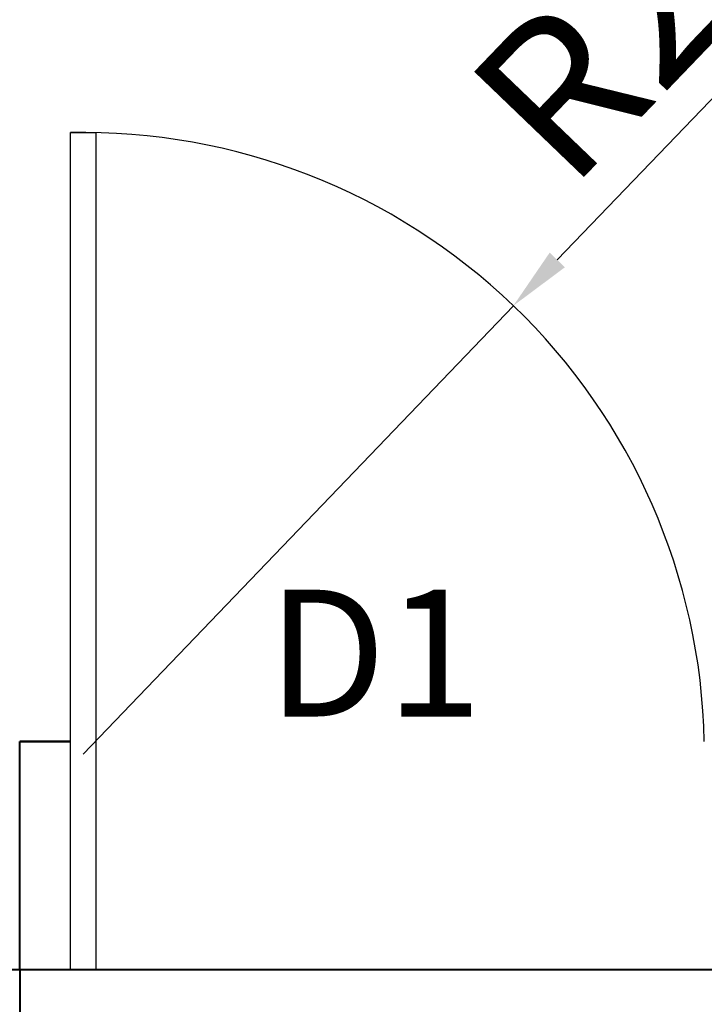
# Model space of a CAD drawing. Units: inches. Extents: x 459864 to 460310, y 324185 to 324787.
# Tile 63 of 112: x 460061 to 460088, y 324282 to 324321. Entities that reach past the tile are written whole.
import ezdxf

# ---------------------------------------------------------------- set-up
doc = ezdxf.new("R2010")
doc.units = ezdxf.units.IN
for name, color, linetype, lineweight in [('A-ANNO-DIMS', 2, 'Continuous', 18), ('A-ANNO-TEXT', 7, 'Continuous', 18), ('A-DOOR', 3, 'Continuous', 25), ('A-WALL', 7, 'Continuous', 40), ('L-SITE-PATT', 252, 'Continuous', 13)]:
    doc.layers.add(name, color=color, linetype=linetype, lineweight=lineweight)
doc.styles.get("Standard").update_dxf_attribs({"font": 'arial.ttf'})
doc.dimstyles.new('ISO-25', dxfattribs={"dimtxt": 6, "dimasz": 2.5, "dimexe": 1.25, "dimexo": 0.625, "dimtad": 1, "dimdec": 1, "dimlunit": 3, "dimtxsty": 'Standard', "dimcen": 2.5, "dimadec": 0, "dimazin": 0, "dimtfac": 1, "dimtdec": 1, "dimtmove": 0, "dimatfit": 3, "dimfxl": 1, "dimarcsym": 0})

# ---------------------------------------------------------------- blocks, each defined once
blk = doc.blocks.new('*D69')
at = {"layer": 'A-ANNO-DIMS', "color": 0, "lineweight": -2, "transparency": 16777216}
for p, q in [((460055.99, 324376.483), (459874.965, 324376.483)), ((459876.215, 324373.983), (459876.215, 324285.983)), ((460060.49, 324283.483), (459874.965, 324283.483))]:
    blk.add_line(p, q, dxfattribs=at)
at = {"layer": 'A-ANNO-DIMS', "color": 0, "transparency": 16777216}
for points in [[(459875.798, 324373.983), (459876.632, 324373.983), (459876.215, 324376.483)], [(459875.798, 324285.983), (459876.632, 324285.983), (459876.215, 324283.483)]]:
    blk.add_solid(points, dxfattribs=at)
at = {"layer": 'Defpoints', "color": 0, "transparency": 16777216}
for p in [(460056.615, 324376.483), (459876.215, 324283.483), (460061.115, 324283.483)]:
    blk.add_point(p, dxfattribs=at)
at = {"layer": 'A-ANNO-DIMS', "color": 0, "transparency": 16777216, "insert": (459872.526, 324329.983), "char_height": 6, "attachment_point": 5, "rotation": 90}
blk.add_mtext('7\'-9"', dxfattribs=at)
blk = doc.blocks.new('*D73')
at = {"layer": 'A-ANNO-DIMS', "color": 0, "lineweight": -2, "transparency": 16777216}
for p, q in [((460109.617, 324339.904), (460082.316, 324311.465)), ((460063.615, 324291.983), (460080.585, 324309.661))]:
    blk.add_line(p, q, dxfattribs=at)
at = {"layer": 'A-ANNO-DIMS', "color": 0, "transparency": 16777216}
blk.add_solid([(460082.016, 324311.753), (460082.617, 324311.176), (460080.585, 324309.661)], dxfattribs=at)
at = {"layer": 'Defpoints', "color": 0, "transparency": 16777216}
for p in [(460080.585, 324309.661), (460063.615, 324291.983)]:
    blk.add_point(p, dxfattribs=at)
at = {"layer": 'A-ANNO-DIMS', "color": 0, "transparency": 16777216, "insert": (460094.144, 324329.167), "char_height": 6, "attachment_point": 5, "rotation": 46.1701}
blk.add_mtext('R2\'-0 1/2"', dxfattribs=at)

msp = doc.modelspace()

# ---------------------------------------------------------------- hatches: boundary and pattern name
at = {"layer": 'L-SITE-PATT'}
h = msp.add_hatch(dxfattribs=at)
h.set_pattern_fill('DOTS', color=256)
h.paths.add_polyline_path([(460269.804, 324283.483), (460247.115, 324283.483), (460121.929, 324283.483), (460121.929, 324252.473), (460117.429, 324252.473), (460110.124, 324252.473), (460110.124, 324243.287), (460080.83, 324243.287), (460080.83, 324252.473), (460061.115, 324252.473), (460061.115, 324251.882), (460077.909, 324251.882), (460077.909, 324199.483), (460080.83, 324199.483), (460080.83, 324207.553), (460110.124, 324207.553), (460110.124, 324199.483), (460110.813, 324199.483), (460262.115, 324199.483), (460269.804, 324199.483)], flags=17)
edge = h.paths.add_edge_path(flags=0)
edge.add_ellipse((460222.59, 324263.813), major_axis=(-8.485, 8.485), ratio=1, start_angle=405, end_angle=495, ccw=False)
edge.add_line((460214.821, 324254.66), (460214.832, 324254.666))
edge.add_ellipse((460222.59, 324263.813), major_axis=(-8.485, 8.485), ratio=1, start_angle=405, end_angle=495, ccw=False)
edge.add_line((460210.759, 324261.781), (460210.768, 324261.787))
edge.add_ellipse((460222.59, 324263.813), major_axis=(-8.485, 8.485), ratio=1, start_angle=405, end_angle=495, ccw=False)
edge.add_ellipse((460222.59, 324263.813), major_axis=(-8.485, 8.485), ratio=1, start_angle=392.754, end_angle=405, ccw=False)
edge.add_ellipse((460222.59, 324263.813), major_axis=(-8.485, 8.485), ratio=1, start_angle=380.9347, end_angle=392.754, ccw=False)
edge.add_line((460211.337, 324267.985), (460211.34, 324267.985))
edge.add_ellipse((460222.59, 324263.813), major_axis=(-8.485, 8.485), ratio=1, start_angle=380.9347, end_angle=392.754, ccw=False)
edge.add_ellipse((460222.59, 324263.813), major_axis=(-8.485, 8.485), ratio=1, start_angle=347.9015, end_angle=380.9347, ccw=False)
edge.add_ellipse((460222.59, 324263.813), major_axis=(-8.485, 8.485), ratio=1, start_angle=327.0619, end_angle=347.9015, ccw=False)
edge.add_ellipse((460222.59, 324263.813), major_axis=(-8.485, 8.485), ratio=1, start_angle=278.3246, end_angle=327.0619, ccw=False)
edge.add_line((460225.158, 324275.536), (460225.158, 324275.535))
edge.add_ellipse((460222.59, 324263.813), major_axis=(-8.485, 8.485), ratio=1, start_angle=278.3246, end_angle=327.0619, ccw=False)
edge.add_ellipse((460222.59, 324263.813), major_axis=(-8.485, 8.485), ratio=1, start_angle=260.6436, end_angle=278.3246, ccw=False)
edge.add_ellipse((460222.59, 324263.813), major_axis=(-8.485, 8.485), ratio=1, start_angle=225, end_angle=260.6436, ccw=False)
edge.add_line((460234.509, 324265.243), (460234.501, 324265.239))
edge.add_ellipse((460222.59, 324263.813), major_axis=(-8.485, 8.485), ratio=1, start_angle=225, end_angle=260.6436, ccw=False)
edge.add_ellipse((460222.59, 324263.813), major_axis=(-8.485, 8.485), ratio=1, start_angle=495, end_angle=585, ccw=False)
edge.add_line((460234.437, 324261.861), (460234.424, 324261.858))
edge.add_ellipse((460222.59, 324263.813), major_axis=(-8.485, 8.485), ratio=1, start_angle=495, end_angle=585, ccw=False)
edge.add_line((460227.95, 324253.067), (460227.946, 324253.083))
edge.add_ellipse((460222.59, 324263.813), major_axis=(-8.485, 8.485), ratio=1, start_angle=495, end_angle=585, ccw=False)
edge.add_line((460226.223, 324252.369), (460226.211, 324252.38))
edge.add_ellipse((460222.59, 324263.813), major_axis=(-8.485, 8.485), ratio=1, start_angle=495, end_angle=585, ccw=False)
h.paths.add_polyline_path([(460219.651, 324254.347), (460218.461, 324253.545), (460218.275, 324254.789), (460219.642, 324256.542), (460219.625, 324260.848), (460216.11, 324257.333), (460214.35, 324256.978), (460215.416, 324259.356), (460212.524, 324258.496), (460213.137, 324259.93), (460218.507, 324263.813), (460222.59, 324263.813), (460222.59, 324267.807), (460218.176, 324272.212), (460219.026, 324274.639), (460222.59, 324272.811), (460222.59, 324275.423), (460223.057, 324274.825), (460222.675, 324273.492), (460225.912, 324267.135), (460219.625, 324260.848)], flags=0)
edge = h.paths.add_edge_path(flags=0)
edge.add_ellipse((460194.576, 324264.046), major_axis=(-8.485, 8.485), ratio=1, start_angle=495, end_angle=585, ccw=False)
edge.add_line((460199.936, 324253.3), (460199.932, 324253.316))
edge.add_ellipse((460194.576, 324264.046), major_axis=(-8.485, 8.485), ratio=1, start_angle=495, end_angle=585, ccw=False)
edge.add_line((460198.208, 324252.603), (460198.196, 324252.613))
edge.add_ellipse((460194.576, 324264.046), major_axis=(-8.485, 8.485), ratio=1, start_angle=495, end_angle=585, ccw=False)
edge.add_ellipse((460194.576, 324264.046), major_axis=(-8.485, 8.485), ratio=1, start_angle=405, end_angle=495, ccw=False)
edge.add_line((460186.806, 324254.893), (460186.817, 324254.899))
edge.add_ellipse((460194.576, 324264.046), major_axis=(-8.485, 8.485), ratio=1, start_angle=405, end_angle=495, ccw=False)
edge.add_line((460182.744, 324262.014), (460182.753, 324262.02))
edge.add_ellipse((460194.576, 324264.046), major_axis=(-8.485, 8.485), ratio=1, start_angle=405, end_angle=495, ccw=False)
edge.add_ellipse((460194.576, 324264.046), major_axis=(-8.485, 8.485), ratio=1, start_angle=392.754, end_angle=405, ccw=False)
edge.add_ellipse((460194.576, 324264.046), major_axis=(-8.485, 8.485), ratio=1, start_angle=380.9347, end_angle=392.754, ccw=False)
edge.add_line((460183.323, 324268.218), (460183.326, 324268.218))
edge.add_ellipse((460194.576, 324264.046), major_axis=(-8.485, 8.485), ratio=1, start_angle=380.9347, end_angle=392.754, ccw=False)
edge.add_ellipse((460194.576, 324264.046), major_axis=(-8.485, 8.485), ratio=1, start_angle=347.9015, end_angle=380.9347, ccw=False)
edge.add_ellipse((460194.576, 324264.046), major_axis=(-8.485, 8.485), ratio=1, start_angle=327.0619, end_angle=347.9015, ccw=False)
edge.add_ellipse((460194.576, 324264.046), major_axis=(-8.485, 8.485), ratio=1, start_angle=278.3246, end_angle=327.0619, ccw=False)
edge.add_line((460197.144, 324275.769), (460197.143, 324275.768))
edge.add_ellipse((460194.576, 324264.046), major_axis=(-8.485, 8.485), ratio=1, start_angle=278.3246, end_angle=327.0619, ccw=False)
edge.add_ellipse((460194.576, 324264.046), major_axis=(-8.485, 8.485), ratio=1, start_angle=260.6436, end_angle=278.3246, ccw=False)
edge.add_ellipse((460194.576, 324264.046), major_axis=(-8.485, 8.485), ratio=1, start_angle=225, end_angle=260.6436, ccw=False)
edge.add_line((460206.494, 324265.476), (460206.487, 324265.473))
edge.add_ellipse((460194.576, 324264.046), major_axis=(-8.485, 8.485), ratio=1, start_angle=225, end_angle=260.6436, ccw=False)
edge.add_ellipse((460194.576, 324264.046), major_axis=(-8.485, 8.485), ratio=1, start_angle=495, end_angle=585, ccw=False)
edge.add_line((460206.422, 324262.094), (460206.409, 324262.091))
h.paths.add_polyline_path([(460191.61, 324261.081), (460191.637, 324254.58), (460190.447, 324253.778), (460190.261, 324255.023), (460191.628, 324256.775), (460191.61, 324261.081), (460188.096, 324257.566), (460186.335, 324257.211), (460187.402, 324259.589), (460184.509, 324258.729), (460185.123, 324260.163), (460190.493, 324264.046), (460194.576, 324264.046), (460194.576, 324268.04), (460190.161, 324272.446), (460191.011, 324274.872), (460194.576, 324273.044), (460194.576, 324275.657), (460195.043, 324275.058), (460194.661, 324273.725), (460197.897, 324267.368)], flags=0)
edge = h.paths.add_edge_path(flags=0)
edge.add_ellipse((460252.912, 324263.578), major_axis=(-8.485, 8.485), ratio=1, start_angle=405, end_angle=495, ccw=False)
edge.add_line((460241.081, 324261.545), (460241.089, 324261.551))
edge.add_ellipse((460252.912, 324263.578), major_axis=(-8.485, 8.485), ratio=1, start_angle=405, end_angle=495, ccw=False)
edge.add_ellipse((460252.912, 324263.578), major_axis=(-8.485, 8.485), ratio=1, start_angle=392.754, end_angle=405, ccw=False)
edge.add_ellipse((460252.912, 324263.578), major_axis=(-8.485, 8.485), ratio=1, start_angle=380.9347, end_angle=392.754, ccw=False)
edge.add_line((460241.659, 324267.749), (460241.662, 324267.749))
edge.add_ellipse((460252.912, 324263.578), major_axis=(-8.485, 8.485), ratio=1, start_angle=380.9347, end_angle=392.754, ccw=False)
edge.add_ellipse((460252.912, 324263.578), major_axis=(-8.485, 8.485), ratio=1, start_angle=347.9015, end_angle=380.9347, ccw=False)
edge.add_ellipse((460252.912, 324263.578), major_axis=(-8.485, 8.485), ratio=1, start_angle=327.0619, end_angle=347.9015, ccw=False)
edge.add_ellipse((460252.912, 324263.578), major_axis=(-8.485, 8.485), ratio=1, start_angle=278.3246, end_angle=327.0619, ccw=False)
edge.add_line((460255.48, 324275.3), (460255.479, 324275.299))
edge.add_ellipse((460252.912, 324263.578), major_axis=(-8.485, 8.485), ratio=1, start_angle=278.3246, end_angle=327.0619, ccw=False)
edge.add_ellipse((460252.912, 324263.578), major_axis=(-8.485, 8.485), ratio=1, start_angle=260.6436, end_angle=278.3246, ccw=False)
edge.add_ellipse((460252.912, 324263.578), major_axis=(-8.485, 8.485), ratio=1, start_angle=225, end_angle=260.6436, ccw=False)
edge.add_line((460264.83, 324265.007), (460264.823, 324265.004))
edge.add_ellipse((460252.912, 324263.578), major_axis=(-8.485, 8.485), ratio=1, start_angle=225, end_angle=260.6436, ccw=False)
edge.add_ellipse((460252.912, 324263.578), major_axis=(-8.485, 8.485), ratio=1, start_angle=495, end_angle=585, ccw=False)
edge.add_line((460264.758, 324261.626), (460264.745, 324261.622))
edge.add_ellipse((460252.912, 324263.578), major_axis=(-8.485, 8.485), ratio=1, start_angle=495, end_angle=585, ccw=False)
edge.add_line((460258.272, 324252.832), (460258.268, 324252.848))
edge.add_ellipse((460252.912, 324263.578), major_axis=(-8.485, 8.485), ratio=1, start_angle=495, end_angle=585, ccw=False)
edge.add_line((460256.545, 324252.134), (460256.533, 324252.144))
edge.add_ellipse((460252.912, 324263.578), major_axis=(-8.485, 8.485), ratio=1, start_angle=495, end_angle=585, ccw=False)
edge.add_ellipse((460252.912, 324263.578), major_axis=(-8.485, 8.485), ratio=1, start_angle=405, end_angle=495, ccw=False)
edge.add_line((460245.143, 324254.424), (460245.153, 324254.43))
h.paths.add_polyline_path([(460244.672, 324256.742), (460245.738, 324259.12), (460242.846, 324258.26), (460243.459, 324259.694), (460248.829, 324263.578), (460252.912, 324263.578), (460252.912, 324267.571), (460248.497, 324271.977), (460249.348, 324274.403), (460252.912, 324272.576), (460252.912, 324275.188), (460253.379, 324274.589), (460252.997, 324273.257), (460256.233, 324266.899), (460249.946, 324260.612), (460249.973, 324254.111), (460248.783, 324253.309), (460248.597, 324254.554), (460249.964, 324256.306), (460249.946, 324260.612), (460246.432, 324257.097)], flags=0)
edge = h.paths.add_edge_path(flags=0)
edge.add_ellipse((460167.439, 324262.833), major_axis=(-8.485, 8.485), ratio=1, start_angle=495, end_angle=585, ccw=False)
edge.add_line((460172.799, 324252.087), (460172.795, 324252.103))
edge.add_ellipse((460167.439, 324262.833), major_axis=(-8.485, 8.485), ratio=1, start_angle=495, end_angle=585, ccw=False)
edge.add_line((460171.071, 324251.389), (460171.059, 324251.399))
edge.add_ellipse((460167.439, 324262.833), major_axis=(-8.485, 8.485), ratio=1, start_angle=495, end_angle=585, ccw=False)
edge.add_ellipse((460167.439, 324262.833), major_axis=(-8.485, 8.485), ratio=1, start_angle=405, end_angle=495, ccw=False)
edge.add_line((460159.669, 324253.679), (460159.68, 324253.685))
edge.add_ellipse((460167.439, 324262.833), major_axis=(-8.485, 8.485), ratio=1, start_angle=405, end_angle=495, ccw=False)
edge.add_line((460155.607, 324260.8), (460155.616, 324260.806))
edge.add_ellipse((460167.439, 324262.833), major_axis=(-8.485, 8.485), ratio=1, start_angle=405, end_angle=495, ccw=False)
edge.add_ellipse((460167.439, 324262.833), major_axis=(-8.485, 8.485), ratio=1, start_angle=392.754, end_angle=405, ccw=False)
edge.add_ellipse((460167.439, 324262.833), major_axis=(-8.485, 8.485), ratio=1, start_angle=380.9347, end_angle=392.754, ccw=False)
edge.add_line((460156.185, 324267.005), (460156.189, 324267.005))
edge.add_ellipse((460167.439, 324262.833), major_axis=(-8.485, 8.485), ratio=1, start_angle=380.9347, end_angle=392.754, ccw=False)
edge.add_ellipse((460167.439, 324262.833), major_axis=(-8.485, 8.485), ratio=1, start_angle=347.9015, end_angle=380.9347, ccw=False)
edge.add_ellipse((460167.439, 324262.833), major_axis=(-8.485, 8.485), ratio=1, start_angle=327.0619, end_angle=347.9015, ccw=False)
edge.add_ellipse((460167.439, 324262.833), major_axis=(-8.485, 8.485), ratio=1, start_angle=278.3246, end_angle=327.0619, ccw=False)
edge.add_line((460170.007, 324274.556), (460170.006, 324274.554))
edge.add_ellipse((460167.439, 324262.833), major_axis=(-8.485, 8.485), ratio=1, start_angle=278.3246, end_angle=327.0619, ccw=False)
edge.add_ellipse((460167.439, 324262.833), major_axis=(-8.485, 8.485), ratio=1, start_angle=260.6436, end_angle=278.3246, ccw=False)
edge.add_ellipse((460167.439, 324262.833), major_axis=(-8.485, 8.485), ratio=1, start_angle=225, end_angle=260.6436, ccw=False)
edge.add_line((460179.357, 324264.262), (460179.35, 324264.259))
edge.add_ellipse((460167.439, 324262.833), major_axis=(-8.485, 8.485), ratio=1, start_angle=225, end_angle=260.6436, ccw=False)
edge.add_ellipse((460167.439, 324262.833), major_axis=(-8.485, 8.485), ratio=1, start_angle=495, end_angle=585, ccw=False)
edge.add_line((460179.285, 324260.881), (460179.272, 324260.877))
h.paths.add_polyline_path([(460164.473, 324259.867), (460164.5, 324253.366), (460163.31, 324252.565), (460163.124, 324253.809), (460164.491, 324255.561), (460164.473, 324259.867), (460160.958, 324256.353), (460159.198, 324255.998), (460160.265, 324258.375), (460157.372, 324257.515), (460157.986, 324258.949), (460163.356, 324262.833), (460167.439, 324262.833), (460167.439, 324266.826), (460163.024, 324271.232), (460163.874, 324273.659), (460167.439, 324271.831), (460167.439, 324274.443), (460167.905, 324273.844), (460167.524, 324272.512), (460170.76, 324266.154)], flags=0)
edge = h.paths.add_edge_path(flags=0)
edge.add_ellipse((460140.758, 324262.37), major_axis=(-8.485, 8.485), ratio=1, start_angle=495, end_angle=585, ccw=False)
edge.add_line((460146.118, 324251.624), (460146.114, 324251.639))
edge.add_ellipse((460140.758, 324262.37), major_axis=(-8.485, 8.485), ratio=1, start_angle=495, end_angle=585, ccw=False)
edge.add_line((460144.391, 324250.926), (460144.379, 324250.936))
edge.add_ellipse((460140.758, 324262.37), major_axis=(-8.485, 8.485), ratio=1, start_angle=495, end_angle=585, ccw=False)
edge.add_ellipse((460140.758, 324262.37), major_axis=(-8.485, 8.485), ratio=1, start_angle=405, end_angle=495, ccw=False)
edge.add_line((460132.989, 324253.216), (460132.999, 324253.222))
edge.add_ellipse((460140.758, 324262.37), major_axis=(-8.485, 8.485), ratio=1, start_angle=405, end_angle=495, ccw=False)
edge.add_line((460128.927, 324260.337), (460128.935, 324260.343))
edge.add_ellipse((460140.758, 324262.37), major_axis=(-8.485, 8.485), ratio=1, start_angle=405, end_angle=495, ccw=False)
edge.add_ellipse((460140.758, 324262.37), major_axis=(-8.485, 8.485), ratio=1, start_angle=392.754, end_angle=405, ccw=False)
edge.add_ellipse((460140.758, 324262.37), major_axis=(-8.485, 8.485), ratio=1, start_angle=380.9347, end_angle=392.754, ccw=False)
edge.add_line((460129.505, 324266.541), (460129.508, 324266.541))
edge.add_ellipse((460140.758, 324262.37), major_axis=(-8.485, 8.485), ratio=1, start_angle=380.9347, end_angle=392.754, ccw=False)
edge.add_ellipse((460140.758, 324262.37), major_axis=(-8.485, 8.485), ratio=1, start_angle=347.9015, end_angle=380.9347, ccw=False)
edge.add_ellipse((460140.758, 324262.37), major_axis=(-8.485, 8.485), ratio=1, start_angle=327.0619, end_angle=347.9015, ccw=False)
edge.add_ellipse((460140.758, 324262.37), major_axis=(-8.485, 8.485), ratio=1, start_angle=278.3246, end_angle=327.0619, ccw=False)
edge.add_line((460143.326, 324274.092), (460143.325, 324274.091))
edge.add_ellipse((460140.758, 324262.37), major_axis=(-8.485, 8.485), ratio=1, start_angle=278.3246, end_angle=327.0619, ccw=False)
edge.add_ellipse((460140.758, 324262.37), major_axis=(-8.485, 8.485), ratio=1, start_angle=260.6436, end_angle=278.3246, ccw=False)
edge.add_ellipse((460140.758, 324262.37), major_axis=(-8.485, 8.485), ratio=1, start_angle=225, end_angle=260.6436, ccw=False)
edge.add_line((460152.677, 324263.799), (460152.669, 324263.796))
edge.add_ellipse((460140.758, 324262.37), major_axis=(-8.485, 8.485), ratio=1, start_angle=225, end_angle=260.6436, ccw=False)
edge.add_ellipse((460140.758, 324262.37), major_axis=(-8.485, 8.485), ratio=1, start_angle=495, end_angle=585, ccw=False)
edge.add_line((460152.604, 324260.418), (460152.592, 324260.414))
h.paths.add_polyline_path([(460137.792, 324259.404), (460137.819, 324252.903), (460136.629, 324252.101), (460136.443, 324253.346), (460137.81, 324255.098), (460137.792, 324259.404), (460134.278, 324255.889), (460132.518, 324255.534), (460133.584, 324257.912), (460130.692, 324257.052), (460131.305, 324258.486), (460136.675, 324262.37), (460140.758, 324262.37), (460140.758, 324266.363), (460136.343, 324270.769), (460137.194, 324273.195), (460140.758, 324271.367), (460140.758, 324273.98), (460141.225, 324273.381), (460140.843, 324272.049), (460144.079, 324265.691)], flags=0)
h.paths.add_polyline_path([(460110.124, 324227.414), (460080.83, 324227.414), (460080.83, 324235.484), (460110.124, 324235.484)], flags=16)
h.paths.add_polyline_path([(460110.124, 324220.797), (460110.124, 324212.727), (460080.83, 324212.727), (460080.83, 324220.797)], flags=16)
h.paths.add_polyline_path([(460269.804, 324283.483), (460247.115, 324283.483), (460121.929, 324283.483), (460121.929, 324252.473), (460117.429, 324252.473), (460110.124, 324252.473), (460110.124, 324243.287), (460080.83, 324243.287), (460080.83, 324252.473), (460061.115, 324252.473), (460061.115, 324251.882), (460077.909, 324251.882), (460077.909, 324199.483), (460080.83, 324199.483), (460080.83, 324207.553), (460110.124, 324207.553), (460110.124, 324199.483), (460262.115, 324199.483), (460269.804, 324199.483)], flags=17)
h.paths.add_polyline_path([(460219.651, 324254.347), (460218.461, 324253.545), (460218.275, 324254.789), (460219.642, 324256.542), (460219.625, 324260.848), (460216.11, 324257.333), (460214.35, 324256.978), (460215.416, 324259.356), (460212.524, 324258.496), (460213.137, 324259.93), (460218.507, 324263.813), (460222.59, 324263.813), (460220.18, 324266.223), (460215.461, 324265.308), (460211.835, 324266.137), (460216.247, 324267.985), (460218.418, 324267.985), (460222.59, 324263.813), (460222.59, 324267.807), (460218.176, 324272.212), (460219.026, 324274.639), (460222.59, 324272.811), (460222.59, 324275.423), (460223.057, 324274.825), (460222.675, 324273.492), (460225.912, 324267.135), (460222.59, 324263.813), (460231.383, 324263.813), (460228.485, 324262.488), (460224.425, 324261.978), (460228.68, 324257.724), (460228.966, 324254.791), (460227.142, 324256.537), (460227.542, 324254.819), (460227.333, 324253.614), (460222.59, 324259.985), (460222.59, 324255.497), (460221.377, 324256.541), (460220.576, 324261.799), (460219.625, 324260.848)], flags=0)
h.paths.add_polyline_path([(460199.127, 324256.77), (460199.528, 324255.052), (460199.319, 324253.848), (460194.576, 324260.218), (460194.576, 324255.73), (460193.363, 324256.774), (460192.561, 324262.032), (460191.61, 324261.081), (460191.637, 324254.58), (460190.447, 324253.778), (460190.261, 324255.023), (460191.628, 324256.775), (460191.61, 324261.081), (460188.096, 324257.566), (460186.335, 324257.211), (460187.402, 324259.589), (460184.509, 324258.729), (460185.123, 324260.163), (460190.493, 324264.046), (460194.576, 324264.046), (460192.166, 324266.456), (460187.446, 324265.541), (460183.82, 324266.37), (460188.232, 324268.218), (460190.404, 324268.218), (460194.576, 324264.046), (460194.576, 324268.04), (460190.161, 324272.446), (460191.011, 324274.872), (460194.576, 324273.044), (460194.576, 324275.657), (460195.043, 324275.058), (460194.661, 324273.725), (460197.897, 324267.368), (460194.576, 324264.046), (460203.368, 324264.046), (460200.47, 324262.721), (460196.411, 324262.212), (460200.665, 324257.957), (460200.951, 324255.024)], flags=0)
h.paths.add_polyline_path([(460244.672, 324256.742), (460245.738, 324259.12), (460242.846, 324258.26), (460243.459, 324259.694), (460248.829, 324263.578), (460252.912, 324263.578), (460250.502, 324265.987), (460245.783, 324265.072), (460242.156, 324265.901), (460246.568, 324267.749), (460248.74, 324267.749), (460252.912, 324263.578), (460252.912, 324267.571), (460248.497, 324271.977), (460249.348, 324274.403), (460252.912, 324272.576), (460252.912, 324275.188), (460253.379, 324274.589), (460252.997, 324273.257), (460256.233, 324266.899), (460252.912, 324263.578), (460261.705, 324263.578), (460258.806, 324262.252), (460254.747, 324261.743), (460259.002, 324257.488), (460259.288, 324254.555), (460257.463, 324256.301), (460257.864, 324254.583), (460257.655, 324253.379), (460252.912, 324259.749), (460252.912, 324255.261), (460251.699, 324256.305), (460250.897, 324261.563), (460249.946, 324260.612), (460249.973, 324254.111), (460248.783, 324253.309), (460248.597, 324254.554), (460249.964, 324256.306), (460249.946, 324260.612), (460246.432, 324257.097)], flags=0)
h.paths.add_polyline_path([(460173.528, 324256.743), (460173.814, 324253.811), (460171.99, 324255.556), (460172.39, 324253.838), (460172.182, 324252.634), (460167.439, 324259.004), (460167.439, 324254.516), (460166.226, 324255.56), (460165.424, 324260.818), (460164.473, 324259.867), (460164.5, 324253.366), (460163.31, 324252.565), (460163.124, 324253.809), (460164.491, 324255.561), (460164.473, 324259.867), (460160.958, 324256.353), (460159.198, 324255.998), (460160.265, 324258.375), (460157.372, 324257.515), (460157.986, 324258.949), (460163.356, 324262.833), (460167.439, 324262.833), (460165.029, 324265.243), (460160.309, 324264.327), (460156.683, 324265.156), (460161.095, 324267.005), (460163.267, 324267.005), (460167.439, 324262.833), (460167.439, 324266.826), (460163.024, 324271.232), (460163.874, 324273.659), (460167.439, 324271.831), (460167.439, 324274.443), (460167.905, 324273.844), (460167.524, 324272.512), (460170.76, 324266.154), (460167.439, 324262.833), (460176.231, 324262.833), (460173.333, 324261.507), (460169.274, 324260.998)], flags=0)
h.paths.add_polyline_path([(460146.848, 324256.28), (460147.134, 324253.347), (460145.31, 324255.093), (460145.71, 324253.375), (460145.501, 324252.171), (460140.758, 324258.541), (460140.758, 324254.053), (460139.545, 324255.097), (460138.744, 324260.355), (460137.792, 324259.404), (460137.819, 324252.903), (460136.629, 324252.101), (460136.443, 324253.346), (460137.81, 324255.098), (460137.792, 324259.404), (460134.278, 324255.889), (460132.518, 324255.534), (460133.584, 324257.912), (460130.692, 324257.052), (460131.305, 324258.486), (460136.675, 324262.37), (460140.758, 324262.37), (460138.348, 324264.779), (460133.629, 324263.864), (460130.002, 324264.693), (460134.414, 324266.541), (460136.586, 324266.541), (460140.758, 324262.37), (460140.758, 324266.363), (460136.343, 324270.769), (460137.194, 324273.195), (460140.758, 324271.367), (460140.758, 324273.98), (460141.225, 324273.381), (460140.843, 324272.049), (460144.079, 324265.691), (460140.758, 324262.37), (460149.551, 324262.37), (460146.653, 324261.044), (460142.593, 324260.535)], flags=0)
edge = h.paths.add_edge_path()
edge.add_line((460269.804, 324272.549), (460260.881, 324272.549))
edge.add_ellipse((460252.912, 324263.578), major_axis=(-8.485, 8.485), ratio=1, start_angle=260.6436, end_angle=273.3846, ccw=False)
edge.add_line((460262.283, 324271.092), (460262.261, 324271.091))
edge.add_ellipse((460252.912, 324263.578), major_axis=(-8.485, 8.485), ratio=1, start_angle=260.6436, end_angle=273.3846, ccw=False)
edge.add_ellipse((460252.912, 324263.578), major_axis=(-8.485, 8.485), ratio=1, start_angle=225, end_angle=260.6436, ccw=False)
edge.add_line((460263.609, 324269.063), (460263.572, 324269.058))
edge.add_ellipse((460252.912, 324263.578), major_axis=(-8.485, 8.485), ratio=1, start_angle=225, end_angle=260.6436, ccw=False)
edge.add_line((460264.615, 324266.306), (460264.585, 324266.305))
edge.add_ellipse((460252.912, 324263.578), major_axis=(-8.485, 8.485), ratio=1, start_angle=225, end_angle=260.6436, ccw=False)
edge.add_line((460264.83, 324265.007), (460264.823, 324265.004))
edge.add_ellipse((460252.912, 324263.578), major_axis=(-8.485, 8.485), ratio=1, start_angle=225, end_angle=260.6436, ccw=False)
edge.add_ellipse((460252.912, 324263.578), major_axis=(-8.485, 8.485), ratio=1, start_angle=495, end_angle=585, ccw=False)
edge.add_line((460264.758, 324261.626), (460264.745, 324261.622))
edge.add_ellipse((460252.912, 324263.578), major_axis=(-8.485, 8.485), ratio=1, start_angle=495, end_angle=585, ccw=False)
edge.add_line((460263.442, 324257.739), (460263.389, 324257.779))
edge.add_ellipse((460252.912, 324263.578), major_axis=(-8.485, 8.485), ratio=1, start_angle=495, end_angle=585, ccw=False)
edge.add_line((460258.128, 324252.744), (460258.102, 324252.779))
edge.add_ellipse((460252.912, 324263.578), major_axis=(-8.485, 8.485), ratio=1, start_angle=495, end_angle=585, ccw=False)
edge.add_line((460256.545, 324252.134), (460256.533, 324252.144))
edge.add_ellipse((460252.912, 324263.578), major_axis=(-8.485, 8.485), ratio=1, start_angle=495, end_angle=585, ccw=False)
edge.add_ellipse((460252.912, 324263.578), major_axis=(-8.485, 8.485), ratio=1, start_angle=405, end_angle=495, ccw=False)
edge.add_line((460250.594, 324251.78), (460250.605, 324251.82))
edge.add_ellipse((460252.912, 324263.578), major_axis=(-8.485, 8.485), ratio=1, start_angle=405, end_angle=495, ccw=False)
edge.add_line((460245.143, 324254.424), (460245.153, 324254.43))
edge.add_ellipse((460252.912, 324263.578), major_axis=(-8.485, 8.485), ratio=1, start_angle=405, end_angle=495, ccw=False)
edge.add_line((460243.525, 324256.059), (460243.56, 324256.091))
edge.add_ellipse((460252.912, 324263.578), major_axis=(-8.485, 8.485), ratio=1, start_angle=405, end_angle=495, ccw=False)
edge.add_line((460241.44, 324259.893), (460241.522, 324259.896))
edge.add_ellipse((460252.912, 324263.578), major_axis=(-8.485, 8.485), ratio=1, start_angle=405, end_angle=495, ccw=False)
edge.add_line((460241.081, 324261.545), (460241.089, 324261.551))
edge.add_ellipse((460252.912, 324263.578), major_axis=(-8.485, 8.485), ratio=1, start_angle=405, end_angle=495, ccw=False)
edge.add_ellipse((460252.912, 324263.578), major_axis=(-8.485, 8.485), ratio=1, start_angle=392.754, end_angle=405, ccw=False)
edge.add_line((460241.05, 324265.438), (460241.063, 324265.443))
edge.add_ellipse((460252.912, 324263.578), major_axis=(-8.485, 8.485), ratio=1, start_angle=392.754, end_angle=405, ccw=False)
edge.add_ellipse((460252.912, 324263.578), major_axis=(-8.485, 8.485), ratio=1, start_angle=380.9347, end_angle=392.754, ccw=False)
edge.add_line((460241.452, 324267.176), (460241.469, 324267.171))
edge.add_ellipse((460252.912, 324263.578), major_axis=(-8.485, 8.485), ratio=1, start_angle=380.9347, end_angle=392.754, ccw=False)
edge.add_line((460241.659, 324267.749), (460241.662, 324267.749))
edge.add_ellipse((460252.912, 324263.578), major_axis=(-8.485, 8.485), ratio=1, start_angle=380.9347, end_angle=392.754, ccw=False)
edge.add_ellipse((460252.912, 324263.578), major_axis=(-8.485, 8.485), ratio=1, start_angle=356.6154, end_angle=380.9347, ccw=False)
edge.add_line((460244.88, 324272.488), (460244.713, 324272.549))
edge.add_line((460244.713, 324272.549), (460230.817, 324272.549))
edge.add_ellipse((460222.59, 324263.813), major_axis=(-8.485, 8.485), ratio=1, start_angle=260.6436, end_angle=271.7178, ccw=False)
edge.add_ellipse((460222.59, 324263.813), major_axis=(-8.485, 8.485), ratio=1, start_angle=225, end_angle=260.6436, ccw=False)
edge.add_line((460233.287, 324269.299), (460233.25, 324269.294))
edge.add_ellipse((460222.59, 324263.813), major_axis=(-8.485, 8.485), ratio=1, start_angle=225, end_angle=260.6436, ccw=False)
edge.add_line((460234.294, 324266.541), (460234.264, 324266.541))
edge.add_ellipse((460222.59, 324263.813), major_axis=(-8.485, 8.485), ratio=1, start_angle=225, end_angle=260.6436, ccw=False)
edge.add_line((460234.509, 324265.243), (460234.501, 324265.239))
edge.add_ellipse((460222.59, 324263.813), major_axis=(-8.485, 8.485), ratio=1, start_angle=225, end_angle=260.6436, ccw=False)
edge.add_ellipse((460222.59, 324263.813), major_axis=(-8.485, 8.485), ratio=1, start_angle=495, end_angle=585, ccw=False)
edge.add_line((460234.437, 324261.861), (460234.424, 324261.858))
edge.add_ellipse((460222.59, 324263.813), major_axis=(-8.485, 8.485), ratio=1, start_angle=495, end_angle=585, ccw=False)
edge.add_line((460233.121, 324257.975), (460233.068, 324258.015))
edge.add_ellipse((460222.59, 324263.813), major_axis=(-8.485, 8.485), ratio=1, start_angle=495, end_angle=585, ccw=False)
edge.add_line((460227.806, 324252.979), (460227.78, 324253.014))
edge.add_ellipse((460222.59, 324263.813), major_axis=(-8.485, 8.485), ratio=1, start_angle=495, end_angle=585, ccw=False)
edge.add_line((460226.223, 324252.369), (460226.211, 324252.38))
edge.add_ellipse((460222.59, 324263.813), major_axis=(-8.485, 8.485), ratio=1, start_angle=495, end_angle=585, ccw=False)
edge.add_ellipse((460222.59, 324263.813), major_axis=(-8.485, 8.485), ratio=1, start_angle=405, end_angle=495, ccw=False)
edge.add_line((460220.272, 324252.016), (460220.283, 324252.055))
edge.add_ellipse((460222.59, 324263.813), major_axis=(-8.485, 8.485), ratio=1, start_angle=405, end_angle=495, ccw=False)
edge.add_line((460214.821, 324254.66), (460214.832, 324254.666))
edge.add_ellipse((460222.59, 324263.813), major_axis=(-8.485, 8.485), ratio=1, start_angle=405, end_angle=495, ccw=False)
edge.add_line((460213.203, 324256.295), (460213.239, 324256.327))
edge.add_ellipse((460222.59, 324263.813), major_axis=(-8.485, 8.485), ratio=1, start_angle=405, end_angle=495, ccw=False)
edge.add_line((460211.118, 324260.128), (460211.201, 324260.131))
edge.add_ellipse((460222.59, 324263.813), major_axis=(-8.485, 8.485), ratio=1, start_angle=405, end_angle=495, ccw=False)
edge.add_line((460210.759, 324261.781), (460210.768, 324261.787))
edge.add_ellipse((460222.59, 324263.813), major_axis=(-8.485, 8.485), ratio=1, start_angle=405, end_angle=495, ccw=False)
edge.add_ellipse((460222.59, 324263.813), major_axis=(-8.485, 8.485), ratio=1, start_angle=392.754, end_angle=405, ccw=False)
edge.add_line((460210.729, 324265.673), (460210.741, 324265.678))
edge.add_ellipse((460222.59, 324263.813), major_axis=(-8.485, 8.485), ratio=1, start_angle=392.754, end_angle=405, ccw=False)
edge.add_ellipse((460222.59, 324263.813), major_axis=(-8.485, 8.485), ratio=1, start_angle=380.9347, end_angle=392.754, ccw=False)
edge.add_line((460211.13, 324267.412), (460211.147, 324267.407))
edge.add_ellipse((460222.59, 324263.813), major_axis=(-8.485, 8.485), ratio=1, start_angle=380.9347, end_angle=392.754, ccw=False)
edge.add_line((460211.337, 324267.985), (460211.34, 324267.985))
edge.add_ellipse((460222.59, 324263.813), major_axis=(-8.485, 8.485), ratio=1, start_angle=380.9347, end_angle=392.754, ccw=False)
edge.add_ellipse((460222.59, 324263.813), major_axis=(-8.485, 8.485), ratio=1, start_angle=358.2822, end_angle=380.9347, ccw=False)
edge.add_line((460213.705, 324271.902), (460213.709, 324271.869))
edge.add_ellipse((460222.59, 324263.813), major_axis=(-8.485, 8.485), ratio=1, start_angle=358.2822, end_angle=380.9347, ccw=False)
edge.add_line((460214.363, 324272.549), (460203.078, 324272.549))
edge.add_line((460203.078, 324272.549), (460203.06, 324272.531))
edge.add_ellipse((460194.576, 324264.046), major_axis=(-8.485, 8.485), ratio=1, start_angle=260.6436, end_angle=270.1168, ccw=False)
edge.add_line((460203.957, 324271.561), (460203.921, 324271.56))
edge.add_ellipse((460194.576, 324264.046), major_axis=(-8.485, 8.485), ratio=1, start_angle=260.6436, end_angle=270.1168, ccw=False)
edge.add_ellipse((460194.576, 324264.046), major_axis=(-8.485, 8.485), ratio=1, start_angle=225, end_angle=260.6436, ccw=False)
edge.add_line((460205.272, 324269.532), (460205.235, 324269.527))
edge.add_ellipse((460194.576, 324264.046), major_axis=(-8.485, 8.485), ratio=1, start_angle=225, end_angle=260.6436, ccw=False)
edge.add_line((460206.279, 324266.774), (460206.249, 324266.774))
edge.add_ellipse((460194.576, 324264.046), major_axis=(-8.485, 8.485), ratio=1, start_angle=225, end_angle=260.6436, ccw=False)
edge.add_line((460206.494, 324265.476), (460206.487, 324265.473))
edge.add_ellipse((460194.576, 324264.046), major_axis=(-8.485, 8.485), ratio=1, start_angle=225, end_angle=260.6436, ccw=False)
edge.add_ellipse((460194.576, 324264.046), major_axis=(-8.485, 8.485), ratio=1, start_angle=495, end_angle=585, ccw=False)
edge.add_line((460206.422, 324262.094), (460206.409, 324262.091))
edge.add_ellipse((460194.576, 324264.046), major_axis=(-8.485, 8.485), ratio=1, start_angle=495, end_angle=585, ccw=False)
edge.add_line((460205.106, 324258.208), (460205.053, 324258.248))
edge.add_ellipse((460194.576, 324264.046), major_axis=(-8.485, 8.485), ratio=1, start_angle=495, end_angle=585, ccw=False)
edge.add_line((460199.792, 324253.212), (460199.766, 324253.248))
edge.add_ellipse((460194.576, 324264.046), major_axis=(-8.485, 8.485), ratio=1, start_angle=495, end_angle=585, ccw=False)
edge.add_line((460198.208, 324252.603), (460198.196, 324252.613))
edge.add_ellipse((460194.576, 324264.046), major_axis=(-8.485, 8.485), ratio=1, start_angle=495, end_angle=585, ccw=False)
edge.add_ellipse((460194.576, 324264.046), major_axis=(-8.485, 8.485), ratio=1, start_angle=405, end_angle=495, ccw=False)
edge.add_line((460192.258, 324252.249), (460192.268, 324252.289))
edge.add_ellipse((460194.576, 324264.046), major_axis=(-8.485, 8.485), ratio=1, start_angle=405, end_angle=495, ccw=False)
edge.add_line((460186.806, 324254.893), (460186.817, 324254.899))
edge.add_ellipse((460194.576, 324264.046), major_axis=(-8.485, 8.485), ratio=1, start_angle=405, end_angle=495, ccw=False)
edge.add_line((460185.188, 324256.528), (460185.224, 324256.56))
edge.add_ellipse((460194.576, 324264.046), major_axis=(-8.485, 8.485), ratio=1, start_angle=405, end_angle=495, ccw=False)
edge.add_line((460183.104, 324260.362), (460183.186, 324260.365))
edge.add_ellipse((460194.576, 324264.046), major_axis=(-8.485, 8.485), ratio=1, start_angle=405, end_angle=495, ccw=False)
edge.add_line((460182.744, 324262.014), (460182.753, 324262.02))
edge.add_ellipse((460194.576, 324264.046), major_axis=(-8.485, 8.485), ratio=1, start_angle=405, end_angle=495, ccw=False)
edge.add_ellipse((460194.576, 324264.046), major_axis=(-8.485, 8.485), ratio=1, start_angle=392.754, end_angle=405, ccw=False)
edge.add_line((460182.714, 324265.906), (460182.726, 324265.912))
edge.add_ellipse((460194.576, 324264.046), major_axis=(-8.485, 8.485), ratio=1, start_angle=392.754, end_angle=405, ccw=False)
edge.add_ellipse((460194.576, 324264.046), major_axis=(-8.485, 8.485), ratio=1, start_angle=380.9347, end_angle=392.754, ccw=False)
edge.add_line((460183.116, 324267.645), (460183.133, 324267.64))
edge.add_ellipse((460194.576, 324264.046), major_axis=(-8.485, 8.485), ratio=1, start_angle=380.9347, end_angle=392.754, ccw=False)
edge.add_line((460183.323, 324268.218), (460183.326, 324268.218))
edge.add_ellipse((460194.576, 324264.046), major_axis=(-8.485, 8.485), ratio=1, start_angle=380.9347, end_angle=392.754, ccw=False)
edge.add_ellipse((460194.576, 324264.046), major_axis=(-8.485, 8.485), ratio=1, start_angle=359.8832, end_angle=380.9347, ccw=False)
edge.add_line((460184.491, 324270.611), (460184.553, 324270.611))
edge.add_ellipse((460194.576, 324264.046), major_axis=(-8.485, 8.485), ratio=1, start_angle=359.8832, end_angle=380.9347, ccw=False)
edge.add_line((460185.346, 324271.76), (460185.379, 324271.728))
edge.add_ellipse((460194.576, 324264.046), major_axis=(-8.485, 8.485), ratio=1, start_angle=359.8832, end_angle=380.9347, ccw=False)
edge.add_line((460185.697, 324272.086), (460185.633, 324272.549))
edge.add_line((460185.633, 324272.549), (460174.683, 324272.549))
edge.add_line((460174.683, 324272.549), (460174.606, 324272.457))
edge.add_ellipse((460167.439, 324262.833), major_axis=(-8.485, 8.485), ratio=1, start_angle=260.6436, end_angle=278.3246, ccw=False)
edge.add_ellipse((460167.439, 324262.833), major_axis=(-8.485, 8.485), ratio=1, start_angle=225, end_angle=260.6436, ccw=False)
edge.add_line((460178.135, 324268.318), (460178.098, 324268.313))
edge.add_ellipse((460167.439, 324262.833), major_axis=(-8.485, 8.485), ratio=1, start_angle=225, end_angle=260.6436, ccw=False)
edge.add_line((460179.142, 324265.561), (460179.112, 324265.56))
edge.add_ellipse((460167.439, 324262.833), major_axis=(-8.485, 8.485), ratio=1, start_angle=225, end_angle=260.6436, ccw=False)
edge.add_line((460179.357, 324264.262), (460179.35, 324264.259))
edge.add_ellipse((460167.439, 324262.833), major_axis=(-8.485, 8.485), ratio=1, start_angle=225, end_angle=260.6436, ccw=False)
edge.add_ellipse((460167.439, 324262.833), major_axis=(-8.485, 8.485), ratio=1, start_angle=495, end_angle=585, ccw=False)
edge.add_line((460179.285, 324260.881), (460179.272, 324260.877))
edge.add_ellipse((460167.439, 324262.833), major_axis=(-8.485, 8.485), ratio=1, start_angle=495, end_angle=585, ccw=False)
edge.add_line((460177.969, 324256.994), (460177.916, 324257.034))
edge.add_ellipse((460167.439, 324262.833), major_axis=(-8.485, 8.485), ratio=1, start_angle=495, end_angle=585, ccw=False)
edge.add_line((460172.655, 324251.999), (460172.629, 324252.034))
edge.add_ellipse((460167.439, 324262.833), major_axis=(-8.485, 8.485), ratio=1, start_angle=495, end_angle=585, ccw=False)
edge.add_line((460171.071, 324251.389), (460171.059, 324251.399))
edge.add_ellipse((460167.439, 324262.833), major_axis=(-8.485, 8.485), ratio=1, start_angle=495, end_angle=585, ccw=False)
edge.add_ellipse((460167.439, 324262.833), major_axis=(-8.485, 8.485), ratio=1, start_angle=405, end_angle=495, ccw=False)
edge.add_line((460165.121, 324251.036), (460165.131, 324251.075))
edge.add_ellipse((460167.439, 324262.833), major_axis=(-8.485, 8.485), ratio=1, start_angle=405, end_angle=495, ccw=False)
edge.add_line((460159.669, 324253.679), (460159.68, 324253.685))
edge.add_ellipse((460167.439, 324262.833), major_axis=(-8.485, 8.485), ratio=1, start_angle=405, end_angle=495, ccw=False)
edge.add_line((460158.051, 324255.314), (460158.087, 324255.347))
edge.add_ellipse((460167.439, 324262.833), major_axis=(-8.485, 8.485), ratio=1, start_angle=405, end_angle=495, ccw=False)
edge.add_line((460155.967, 324259.148), (460156.049, 324259.151))
edge.add_ellipse((460167.439, 324262.833), major_axis=(-8.485, 8.485), ratio=1, start_angle=405, end_angle=495, ccw=False)
edge.add_line((460155.607, 324260.8), (460155.616, 324260.806))
edge.add_ellipse((460167.439, 324262.833), major_axis=(-8.485, 8.485), ratio=1, start_angle=405, end_angle=495, ccw=False)
edge.add_ellipse((460167.439, 324262.833), major_axis=(-8.485, 8.485), ratio=1, start_angle=392.754, end_angle=405, ccw=False)
edge.add_line((460155.577, 324264.693), (460155.589, 324264.698))
edge.add_ellipse((460167.439, 324262.833), major_axis=(-8.485, 8.485), ratio=1, start_angle=392.754, end_angle=405, ccw=False)
edge.add_ellipse((460167.439, 324262.833), major_axis=(-8.485, 8.485), ratio=1, start_angle=380.9347, end_angle=392.754, ccw=False)
edge.add_line((460155.979, 324266.432), (460155.996, 324266.426))
edge.add_ellipse((460167.439, 324262.833), major_axis=(-8.485, 8.485), ratio=1, start_angle=380.9347, end_angle=392.754, ccw=False)
edge.add_line((460156.185, 324267.005), (460156.189, 324267.005))
edge.add_ellipse((460167.439, 324262.833), major_axis=(-8.485, 8.485), ratio=1, start_angle=380.9347, end_angle=392.754, ccw=False)
edge.add_ellipse((460167.439, 324262.833), major_axis=(-8.485, 8.485), ratio=1, start_angle=350.9345, end_angle=380.9347, ccw=False)
edge.add_line((460157.363, 324269.397), (460157.414, 324269.397))
edge.add_ellipse((460167.439, 324262.833), major_axis=(-8.485, 8.485), ratio=1, start_angle=350.9345, end_angle=380.9347, ccw=False)
edge.add_line((460158.221, 324270.535), (460158.236, 324270.519))
edge.add_ellipse((460167.439, 324262.833), major_axis=(-8.485, 8.485), ratio=1, start_angle=350.9345, end_angle=380.9347, ccw=False)
edge.add_line((460159.379, 324271.753), (460159.419, 324271.738))
edge.add_ellipse((460167.439, 324262.833), major_axis=(-8.485, 8.485), ratio=1, start_angle=350.9345, end_angle=380.9347, ccw=False)
edge.add_line((460160.396, 324272.549), (460147.112, 324272.549))
edge.add_ellipse((460140.758, 324262.37), major_axis=(-8.485, 8.485), ratio=1, start_angle=278.3246, end_angle=283.0261, ccw=False)
edge.add_ellipse((460140.758, 324262.37), major_axis=(-8.485, 8.485), ratio=1, start_angle=260.6436, end_angle=278.3246, ccw=False)
edge.add_ellipse((460140.758, 324262.37), major_axis=(-8.485, 8.485), ratio=1, start_angle=225, end_angle=260.6436, ccw=False)
edge.add_line((460151.455, 324267.855), (460151.418, 324267.85))
edge.add_ellipse((460140.758, 324262.37), major_axis=(-8.485, 8.485), ratio=1, start_angle=225, end_angle=260.6436, ccw=False)
edge.add_line((460152.462, 324265.098), (460152.431, 324265.097))
edge.add_ellipse((460140.758, 324262.37), major_axis=(-8.485, 8.485), ratio=1, start_angle=225, end_angle=260.6436, ccw=False)
edge.add_line((460152.677, 324263.799), (460152.669, 324263.796))
edge.add_ellipse((460140.758, 324262.37), major_axis=(-8.485, 8.485), ratio=1, start_angle=225, end_angle=260.6436, ccw=False)
edge.add_ellipse((460140.758, 324262.37), major_axis=(-8.485, 8.485), ratio=1, start_angle=495, end_angle=585, ccw=False)
edge.add_line((460152.604, 324260.418), (460152.592, 324260.414))
edge.add_ellipse((460140.758, 324262.37), major_axis=(-8.485, 8.485), ratio=1, start_angle=495, end_angle=585, ccw=False)
edge.add_line((460151.288, 324256.531), (460151.235, 324256.571))
edge.add_ellipse((460140.758, 324262.37), major_axis=(-8.485, 8.485), ratio=1, start_angle=495, end_angle=585, ccw=False)
edge.add_line((460145.974, 324251.535), (460145.948, 324251.571))
edge.add_ellipse((460140.758, 324262.37), major_axis=(-8.485, 8.485), ratio=1, start_angle=495, end_angle=585, ccw=False)
edge.add_line((460144.391, 324250.926), (460144.379, 324250.936))
edge.add_ellipse((460140.758, 324262.37), major_axis=(-8.485, 8.485), ratio=1, start_angle=495, end_angle=585, ccw=False)
edge.add_ellipse((460140.758, 324262.37), major_axis=(-8.485, 8.485), ratio=1, start_angle=405, end_angle=495, ccw=False)
edge.add_line((460138.44, 324250.572), (460138.451, 324250.612))
edge.add_ellipse((460140.758, 324262.37), major_axis=(-8.485, 8.485), ratio=1, start_angle=405, end_angle=495, ccw=False)
edge.add_line((460132.989, 324253.216), (460132.999, 324253.222))
edge.add_ellipse((460140.758, 324262.37), major_axis=(-8.485, 8.485), ratio=1, start_angle=405, end_angle=495, ccw=False)
edge.add_line((460131.371, 324254.851), (460131.406, 324254.883))
edge.add_ellipse((460140.758, 324262.37), major_axis=(-8.485, 8.485), ratio=1, start_angle=405, end_angle=495, ccw=False)
edge.add_line((460129.286, 324258.685), (460129.369, 324258.688))
edge.add_ellipse((460140.758, 324262.37), major_axis=(-8.485, 8.485), ratio=1, start_angle=405, end_angle=495, ccw=False)
edge.add_line((460128.927, 324260.337), (460128.935, 324260.343))
edge.add_ellipse((460140.758, 324262.37), major_axis=(-8.485, 8.485), ratio=1, start_angle=405, end_angle=495, ccw=False)
edge.add_ellipse((460140.758, 324262.37), major_axis=(-8.485, 8.485), ratio=1, start_angle=392.754, end_angle=405, ccw=False)
edge.add_line((460128.896, 324264.23), (460128.909, 324264.235))
edge.add_ellipse((460140.758, 324262.37), major_axis=(-8.485, 8.485), ratio=1, start_angle=392.754, end_angle=405, ccw=False)
edge.add_ellipse((460140.758, 324262.37), major_axis=(-8.485, 8.485), ratio=1, start_angle=380.9347, end_angle=392.754, ccw=False)
edge.add_line((460129.298, 324265.968), (460129.315, 324265.963))
edge.add_ellipse((460140.758, 324262.37), major_axis=(-8.485, 8.485), ratio=1, start_angle=380.9347, end_angle=392.754, ccw=False)
edge.add_line((460129.505, 324266.541), (460129.508, 324266.541))
edge.add_ellipse((460140.758, 324262.37), major_axis=(-8.485, 8.485), ratio=1, start_angle=380.9347, end_angle=392.754, ccw=False)
edge.add_ellipse((460140.758, 324262.37), major_axis=(-8.485, 8.485), ratio=1, start_angle=347.9015, end_angle=380.9347, ccw=False)
edge.add_line((460130.697, 324268.934), (460130.727, 324268.934))
edge.add_ellipse((460140.758, 324262.37), major_axis=(-8.485, 8.485), ratio=1, start_angle=347.9015, end_angle=380.9347, ccw=False)
edge.add_line((460131.869, 324270.48), (460131.879, 324270.413))
edge.add_ellipse((460140.758, 324262.37), major_axis=(-8.485, 8.485), ratio=1, start_angle=347.9015, end_angle=380.9347, ccw=False)
edge.add_line((460132.734, 324271.277), (460132.705, 324271.287))
edge.add_ellipse((460140.758, 324262.37), major_axis=(-8.485, 8.485), ratio=1, start_angle=347.9015, end_angle=380.9347, ccw=False)
edge.add_line((460134.24, 324272.445), (460134.204, 324272.549))
edge.add_line((460134.204, 324272.549), (460121.929, 324272.549))
edge.add_line((460121.929, 324272.549), (460121.929, 324252.473))
edge.add_line((460121.929, 324252.473), (460117.429, 324252.473))
edge.add_line((460117.429, 324252.473), (460110.124, 324252.473))
edge.add_line((460110.124, 324252.473), (460110.124, 324243.287))
edge.add_line((460110.124, 324243.287), (460080.83, 324243.287))
edge.add_line((460080.83, 324243.287), (460080.83, 324252.473))
edge.add_line((460080.83, 324252.473), (460061.115, 324252.473))
edge.add_line((460061.115, 324252.473), (460061.115, 324251.882))
edge.add_line((460061.115, 324251.882), (460077.909, 324251.882))
edge.add_line((460077.909, 324251.882), (460077.909, 324199.483))
edge.add_line((460077.909, 324199.483), (460080.83, 324199.483))
edge.add_line((460080.83, 324199.483), (460080.83, 324207.553))
edge.add_line((460080.83, 324207.553), (460110.124, 324207.553))
edge.add_line((460110.124, 324207.553), (460110.124, 324199.483))
edge.add_line((460110.124, 324199.483), (460110.813, 324199.483))
edge.add_line((460110.813, 324199.483), (460262.115, 324199.483))
edge.add_line((460262.115, 324199.483), (460269.804, 324199.483))
edge.add_line((460269.804, 324199.483), (460269.804, 324272.549))

# ---------------------------------------------------------------- linework, layer by layer
at = {"layer": 'A-DOOR'}
for p, q in [((460063.115, 324283.483), (460063.115, 324316.483)), ((460063.115, 324316.483), (460064.115, 324316.483)), ((460064.115, 324316.483), (460064.115, 324283.483))]:
    msp.add_line(p, q, dxfattribs=at)
msp.add_arc((460063.615, 324291.983), 24.505, 1.1691, 91.1691, dxfattribs=at)
at = {"layer": 'A-WALL'}
for p, q in [((460061.115, 324283.483), (460061.115, 324292.483)), ((460061.115, 324292.483), (460063.115, 324292.483)), ((460063.115, 324292.483), (460061.115, 324292.483)), ((460063.115, 324292.483), (460061.115, 324292.483)), ((460061.115, 324283.483), (460056.615, 324283.483)), ((460247.115, 324283.483), (460061.115, 324283.483)), ((460061.115, 324283.483), (460061.115, 324235.483))]:
    msp.add_line(p, q, dxfattribs=at)

# ---------------------------------------------------------------- texts
at = {"layer": 'A-ANNO-TEXT', "insert": (460070.877, 324298.467), "char_height": 5, "attachment_point": 1}
msp.add_mtext('D1', dxfattribs=at)

# ---------------------------------------------------------------- dimensions: what is measured, and where the dimension line sits
at = {"layer": 'A-ANNO-DIMS'}
dim = msp.add_linear_dim(base=(459876.215, 324283.483), p1=(460056.615, 324376.483), p2=(460061.115, 324283.483), angle=90, dimstyle='ISO-25', override={"dimdec": 1, "dimlfac": 1, "dimrnd": 0, "dimzin": 1, "dimdsep": 46, "dimlunit": 4, "dimfrac": 2}, dxfattribs=at)
dim.commit()
dim.dimension.update_dxf_attribs({"geometry": '*D69', "text_midpoint": (459872.526, 324329.983)})
dim = msp.add_radius_dim(center=(460063.615, 324291.983), mpoint=(460080.585, 324309.661), dimstyle='ISO-25', override={"dimdec": 1, "dimlfac": 1, "dimrnd": 0, "dimzin": 1, "dimdsep": 46, "dimlunit": 4, "dimfrac": 2}, dxfattribs=at)
dim.commit()
dim.dimension.update_dxf_attribs({"geometry": '*D73', "text_midpoint": (460094.144, 324329.167)})

doc.saveas('drawing.dxf')
